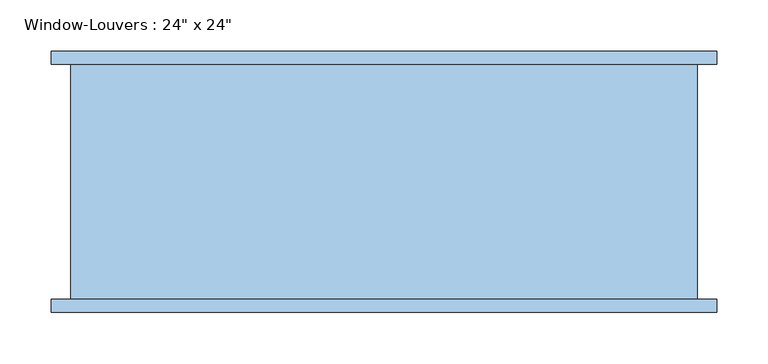
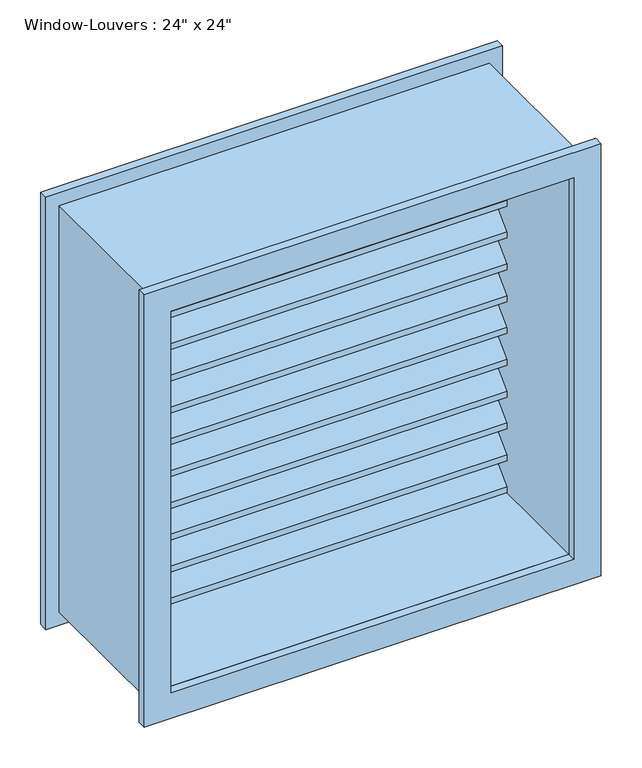
"""IFC4 building model written with IfcOpenShell, lengths in millimetres: window geometry."""

from ifc_helpers import new_model, si_unit, frame, origin, place, context, project, spatial, polyline, outline, extrude, source, transform, mapped, element, save


def window_f2d8fef0(model_context):
    return source(origin(), model_context, "Body", "SweptSolid", [
        extrude(outline(polyline([(107.95, 1419.1754778), (107.95, 1410.1952217), (69.85, 1448.2952217), (31.75, 1410.1952217), (31.75, 1419.1754778), (69.85, 1457.2754778), (107.95, 1419.1754778)])), frame((-285.75, 0.0, 0.0), z_axis=(1.0, 0.0, 0.0), x_axis=(0.0, 1.0, 0.0)), (0.0, 0.0, 1.0), 571.5),
        extrude(outline(polyline([(107.95, 1371.5009557), (107.95, 1362.5206995), (69.85, 1400.6206995), (31.75, 1362.5206995), (31.75, 1371.5009557), (69.85, 1409.6009557), (107.95, 1371.5009557)])), frame((-285.75, 0.0, 0.0), z_axis=(1.0, 0.0, 0.0), x_axis=(0.0, 1.0, 0.0)), (0.0, 0.0, 1.0), 571.5),
        extrude(outline(polyline([(107.95, 1323.8264335), (107.95, 1314.8461774), (69.85, 1352.9461774), (31.75, 1314.8461774), (31.75, 1323.8264335), (69.85, 1361.9264335), (107.95, 1323.8264335)])), frame((-285.75, 0.0, 0.0), z_axis=(1.0, 0.0, 0.0), x_axis=(0.0, 1.0, 0.0)), (0.0, 0.0, 1.0), 571.5),
        extrude(outline(polyline([(107.95, 1276.1519113), (107.95, 1267.1716552), (69.85, 1305.2716552), (31.75, 1267.1716552), (31.75, 1276.1519113), (69.85, 1314.2519113), (107.95, 1276.1519113)])), frame((-285.75, 0.0, 0.0), z_axis=(1.0, 0.0, 0.0), x_axis=(0.0, 1.0, 0.0)), (0.0, 0.0, 1.0), 571.5),
        extrude(outline(polyline([(107.95, 1228.4773891), (107.95, 1219.497133), (69.85, 1257.597133), (31.75, 1219.497133), (31.75, 1228.4773891), (69.85, 1266.5773891), (107.95, 1228.4773891)])), frame((-285.75, 0.0, 0.0), z_axis=(1.0, 0.0, 0.0), x_axis=(0.0, 1.0, 0.0)), (0.0, 0.0, 1.0), 571.5),
        extrude(outline(polyline([(107.95, 1180.802867), (107.95, 1171.8226109), (69.85, 1209.9226109), (31.75, 1171.8226109), (31.75, 1180.802867), (69.85, 1218.902867), (107.95, 1180.802867)])), frame((-285.75, 0.0, 0.0), z_axis=(1.0, 0.0, 0.0), x_axis=(0.0, 1.0, 0.0)), (0.0, 0.0, 1.0), 571.5),
        extrude(outline(polyline([(107.95, 1133.1283448), (107.95, 1124.1480887), (69.85, 1162.2480887), (31.75, 1124.1480887), (31.75, 1133.1283448), (69.85, 1171.2283448), (107.95, 1133.1283448)])), frame((-285.75, 0.0, 0.0), z_axis=(1.0, 0.0, 0.0), x_axis=(0.0, 1.0, 0.0)), (0.0, 0.0, 1.0), 571.5),
        extrude(outline(polyline([(107.95, 1085.4538226), (107.95, 1076.4735665), (69.85, 1114.5735665), (31.75, 1076.4735665), (31.75, 1085.4538226), (69.85, 1123.5538226), (107.95, 1085.4538226)])), frame((-285.75, 0.0, 0.0), z_axis=(1.0, 0.0, 0.0), x_axis=(0.0, 1.0, 0.0)), (0.0, 0.0, 1.0), 571.5),
        extrude(outline(polyline([(107.95, 1037.7793005), (107.95, 1028.7990443), (69.85, 1066.8990443), (31.75, 1028.7990443), (31.75, 1037.7793005), (69.85, 1075.8793005), (107.95, 1037.7793005)])), frame((-285.75, 0.0, 0.0), z_axis=(1.0, 0.0, 0.0), x_axis=(0.0, 1.0, 0.0)), (0.0, 0.0, 1.0), 571.5),
        extrude(outline(polyline([(107.95, 990.1047783), (107.95, 981.1245222), (69.85, 1019.2245222), (31.75, 981.1245222), (31.75, 990.1047783), (69.85, 1028.2047783), (107.95, 990.1047783)])), frame((-285.75, 0.0, 0.0), z_axis=(1.0, 0.0, 0.0), x_axis=(0.0, 1.0, 0.0)), (0.0, 0.0, 1.0), 571.5),
        extrude(outline(polyline([(107.95, 1466.85), (107.95, 1457.8697439), (69.85, 1495.9697439), (31.75, 1457.8697439), (31.75, 1466.85), (69.85, 1504.95), (107.95, 1466.85)])), frame((-285.75, 0.0, 0.0), z_axis=(1.0, 0.0, 0.0), x_axis=(0.0, 1.0, 0.0)), (0.0, 0.0, 1.0), 571.5),
        extrude(outline(polyline([(107.95, 942.4302561), (107.95, 933.45), (69.85, 971.55), (31.75, 933.45), (31.75, 942.4302561), (69.85, 980.5302561), (107.95, 942.4302561)])), frame((-285.75, 0.0, 0.0), z_axis=(1.0, 0.0, 0.0), x_axis=(0.0, 1.0, 0.0)), (0.0, 0.0, 1.0), 571.5),
        extrude(outline(polyline([(1524.0, 304.8), (1524.0, -304.8), (914.4, -304.8), (914.4, 304.8), (1524.0, 304.8)]), holes=[polyline([(1504.95, 285.75), (933.45, 285.75), (933.45, -285.75), (1504.95, -285.75), (1504.95, 285.75)])]), frame((0.0, -120.65, 0.0), z_axis=(0.0, 1.0, 0.0), x_axis=(0.0, 0.0, 1.0)), (0.0, 0.0, 1.0), 228.6),
        extrude(outline(polyline([(1543.05, 323.85), (1543.05, -323.85), (895.35, -323.85), (895.35, 323.85), (1543.05, 323.85)]), holes=[polyline([(1504.95, 285.75), (933.45, 285.75), (933.45, -285.75), (1504.95, -285.75), (1504.95, 285.75)])]), frame((0.0, -133.35, 0.0), z_axis=(0.0, 1.0, 0.0), x_axis=(0.0, 0.0, 1.0)), (0.0, 0.0, 1.0), 12.7),
        extrude(outline(polyline([(1543.05, -323.85), (895.35, -323.85), (895.35, 323.85), (1543.05, 323.85), (1543.05, -323.85)]), holes=[polyline([(1504.95, -285.75), (1504.95, 285.75), (933.45, 285.75), (933.45, -285.75), (1504.95, -285.75)])]), frame((0.0, 107.95, 0.0), z_axis=(0.0, 1.0, 0.0), x_axis=(0.0, 0.0, 1.0)), (0.0, 0.0, 1.0), 12.7),
    ])


if __name__ == "__main__":
    model = new_model("IFC4")
    model_context = context("Model", 3, world=origin())
    ifc_project = project(units=[si_unit("LENGTHUNIT", "METRE", prefix="MILLI")], contexts=[model_context])
    site = spatial("IfcSite", under=ifc_project)
    building = spatial("IfcBuilding", under=site)
    placement = place(None, origin())
    window_shape = window_f2d8fef0(model_context)
    element("IfcWindow", 1, ObjectType="Window-Louvers : 24\" x 24\"", at=placement, inside=building, context=model_context, shape_type="MappedRepresentation", body=[
        mapped(window_shape, transform((0.0, 0.0, 0.0), x_axis=(1.0, 0.0, 0.0), y_axis=(0.0, 1.0, 0.0), z_axis=(0.0, 0.0, 1.0))),
    ])
    save(model, "model.ifc")

# Revit data of these elements
# Type "Window-Louvers : 24\" x 24\""
#   Type Mark = "25"
#   Construction Type Id = "GSP4R"
#   Assembly Code = "B20"
#   Analytic Construction = "1/8 in Pilkington single glazing"
#   Visual Light Transmittance = 0.9
#   Thermal Resistance (R) = 1.53941 (h·ft²·°F)/BTU
#   Solar Heat Gain Coefficient = 0.78
#   Max Height = 1' - 11.74264"
#   Height = 2' - 0"
#   Heat Transfer Coefficient (U) = 0.6496 BTU/(h·ft²·°F)
#   Blade Width [instance default] = 1' - 10 1/2"
#   Blade Vertical Thickness = 0' - 0.35355"
#   Blade Thickness = 0' - 0 1/4"
#   Blade Spacing = 0' - 1 1/2"
#   Blade Height = 0' - 1.85355"
#   Blade Depth = 0' - 3"
#   Blade Angle = 45.00°
#   Default Sill Height = 3' - 0"
#   Trim Projection_Exterior = 0' - 0 1/2"
#   Trim Projection_Interior = 0' - 0 1/2"
#   Trim Width_Exterior = 0' - 1 1/2"
#   Trim Width_Interior = 0' - 1 1/2"
#   Width = 2' - 0"
#   Max Blade Count = 12
#   Define Thermal Properties by = 1
#   Blade Count = 12
#   Frame Material = Birch
#   Louver Material = Birch
#   Trim Exterior Material = Birch
#   Trim Interior Material = Birch
#   Wall Closure = (empty or 0)
# Element 1 (IfcWindow, "Window-Louvers : 24\" x 24\"")
#   Materials on its faces: "Birch"
# Materials
#   "Birch": class "Wood", colour RGB 224 178 126, transparency 0, Description = "Betula Alleghaniensis", Cost = 0
